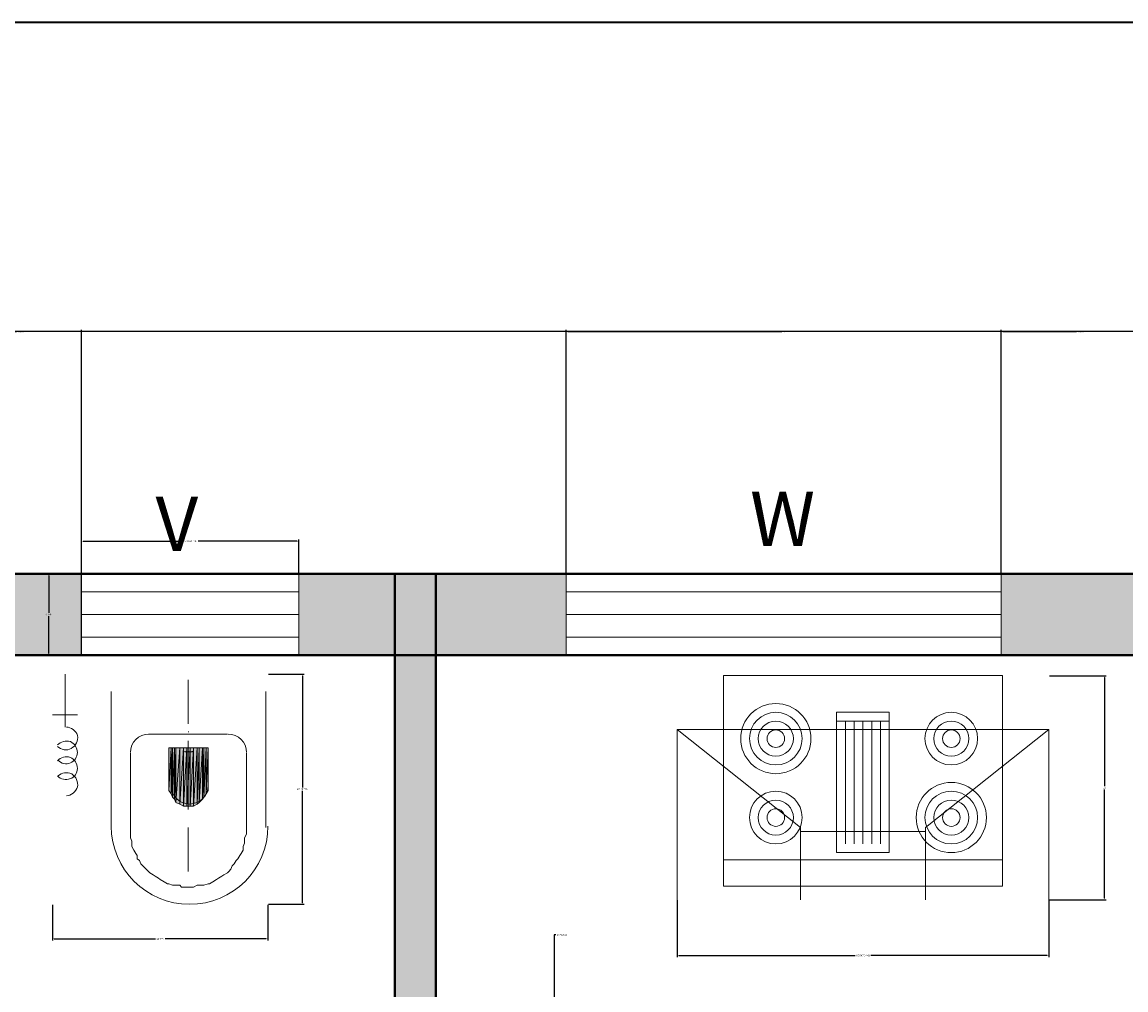
# Model space of a CAD drawing. Units: inches. Extents: x 25176543 to 25177243, y 80295576 to 80296086.
# Tile 9 of 11: x 25176879 to 25177000, y 80295979 to 80296086. Entities that reach past the tile are written whole.
import ezdxf

# ---------------------------------------------------------------- set-up
doc = ezdxf.new("R2010")
doc.units = ezdxf.units.IN
doc.header["$MEASUREMENT"] = 0
for name, color, linetype, lineweight in [('A-ANNO-DIMS', 2, 'Continuous', 18), ('A-ANNO-IDEN', 7, 'Continuous', 18), ('A-ANNO-TTLB', 7, 'Continuous', 35), ('A-EQPM', 8, 'Continuous', 18), ('A-FLOR-FIXT', 8, 'Continuous', 18), ('A-GLAZ', 4, 'Continuous', 18), ('A-WALL', 7, 'Continuous', 40), ('A-WALL-PATT', 146, 'Continuous', 13)]:
    doc.layers.add(name, color=color, linetype=linetype, lineweight=lineweight)
doc.styles.get("Standard").update_dxf_attribs({"font": 'arial.ttf'})
doc.dimstyles.get("Standard").update_dxf_attribs({"dimtxt": 0.18, "dimasz": 0.18, "dimexe": 0.18, "dimexo": 0.0625, "dimgap": 0.09, "dimtad": 0, "dimtih": 1, "dimtoh": 1, "dimdec": 4, "dimzin": 0, "dimdsep": 46, "dimtxsty": 'Standard', "dimcen": 0.09, "dimadec": 0, "dimazin": 0, "dimtfac": 1, "dimtdec": 4, "dimtofl": 0, "dimtmove": 0, "dimatfit": 3, "dimfxl": 1, "dimtolj": 1, "dimtzin": 0, "dimarcsym": 0})

# ---------------------------------------------------------------- blocks, each defined once
blk = doc.blocks.new('chimmne')
for p, q in [((17.89, 6.07), (-18.11, 6.07)), ((-18.11, 6.07), (-18.11, -10.43)), ((-6.16, -3.43), (-18.11, 6.07)), ((5.94, -3.43), (17.89, 6.07)), ((17.89, 6.07), (17.89, -10.43)), ((-6.16, -3.43), (-6.16, -10.43)), ((5.94, -3.82), (-6.16, -3.82)), ((5.94, -3.43), (5.94, -10.43))]:
    blk.add_line(p, q)
for points in [[(-13.61, -9.12), (-13.61, 11.28), (13.39, 11.28), (13.39, -9.12)], [(-2.66, -5.87), (-2.66, 7.73), (2.44, 7.73), (2.44, -5.87)]]:
    blk.add_lwpolyline(points, close=True)
for points in [[(-2.66, 6.88), (2.44, 6.88)], [(-1.81, 6.88), (-1.81, -5.02)], [(-0.96, -5.02), (-0.96, 6.88)], [(-0.11, 6.88), (-0.11, -5.02)], [(0.74, -5.02), (0.74, 6.88)], [(1.59, 6.88), (1.59, -5.02)], [(13.39, -6.57), (-13.61, -6.57)]]:
    blk.add_lwpolyline(points)
for centre, radius in [((-8.55, 5.18), 3.4), ((-8.55, 5.18), 2.55), ((8.44, 5.18), 2.55), ((-8.55, 5.18), 1.7), ((8.44, 5.18), 1.7), ((-8.55, 5.18), 0.85), ((8.44, 5.18), 0.85), ((-8.55, -2.47), 2.55), ((8.44, -2.47), 3.4), ((8.44, -2.47), 2.55), ((-8.55, -2.47), 1.7), ((8.44, -2.47), 1.7), ((-8.55, -2.47), 0.85), ((8.44, -2.47), 0.85)]:
    blk.add_circle(centre, radius)
blk = doc.blocks.new('WC-PLAN')
h = blk.add_hatch(color=256)
h.paths.add_polyline_path([(12.84, 17.3), (12.84, 12.59), (13.07, 17.3)])
h.paths.add_polyline_path([(12.84, 12.59), (13.07, 17.3), (13.07, 12.21)])
h = blk.add_hatch(color=256)
h.paths.add_polyline_path([(13.07, 17.3), (13.07, 12.21), (13.22, 17.3)])
h.paths.add_polyline_path([(13.07, 12.21), (13.22, 17.3), (13.22, 11.83)])
h = blk.add_hatch(color=256)
h.paths.add_polyline_path([(13.22, 17.3), (13.22, 11.83), (13.45, 17.3)])
h.paths.add_polyline_path([(13.22, 11.83), (13.45, 17.3), (13.45, 11.61)])
h = blk.add_hatch(color=256)
h.paths.add_polyline_path([(13.45, 17.3), (13.45, 11.61), (13.6, 17.3)])
h.paths.add_polyline_path([(13.45, 11.61), (13.6, 17.3), (13.6, 11.23)])
h = blk.add_hatch(color=256)
h.paths.add_polyline_path([(13.6, 17.3), (13.6, 11.23), (14.06, 17.3)])
h.paths.add_polyline_path([(13.6, 11.23), (14.06, 17.3), (14.06, 11.08)])
h = blk.add_hatch(color=256)
h.paths.add_polyline_path([(14.06, 17.3), (14.06, 11.08), (14.44, 17.3)])
h.paths.add_polyline_path([(14.06, 11.08), (14.44, 17.3), (14.44, 10.85)])
h = blk.add_hatch(color=256)
h.paths.add_polyline_path([(14.44, 17.3), (14.44, 10.85), (14.81, 17.3)])
h.paths.add_polyline_path([(14.44, 10.85), (14.81, 17.3), (14.81, 10.85)])
h = blk.add_hatch(color=256)
h.paths.add_polyline_path([(14.81, 17.3), (14.81, 10.85), (15.19, 17.3)])
h.paths.add_polyline_path([(14.81, 10.85), (15.19, 17.3), (15.19, 10.85)])
h = blk.add_hatch(color=256)
h.paths.add_polyline_path([(15.19, 17.3), (15.19, 10.85), (15.57, 17.3)])
h.paths.add_polyline_path([(15.19, 10.85), (15.57, 17.3), (15.57, 10.85)])
h = blk.add_hatch(color=256)
h.paths.add_polyline_path([(15.57, 17.3), (15.57, 10.85), (15.95, 17.3)])
h.paths.add_polyline_path([(15.57, 10.85), (15.95, 17.3), (15.95, 11.08)])
h = blk.add_hatch(color=256)
h.paths.add_polyline_path([(15.95, 17.3), (15.95, 11.08), (16.18, 17.3)])
h.paths.add_polyline_path([(15.95, 11.08), (16.18, 17.3), (16.18, 11.23)])
h = blk.add_hatch(color=256)
h.paths.add_polyline_path([(16.18, 17.3), (16.18, 11.23), (16.56, 17.3)])
h.paths.add_polyline_path([(16.18, 11.23), (16.56, 17.3), (16.56, 11.61)])
h = blk.add_hatch(color=256)
h.paths.add_polyline_path([(16.56, 17.3), (16.56, 11.61), (16.71, 17.3)])
h.paths.add_polyline_path([(16.56, 11.61), (16.71, 17.3), (16.71, 11.83)])
h = blk.add_hatch(color=256)
h.paths.add_polyline_path([(16.71, 17.3), (16.71, 11.83), (16.94, 17.3)])
h.paths.add_polyline_path([(16.71, 11.83), (16.94, 17.3), (16.94, 12.21)])
h = blk.add_hatch(color=256)
h.paths.add_polyline_path([(16.94, 17.3), (16.94, 12.21), (17.17, 17.3)])
h.paths.add_polyline_path([(16.94, 12.21), (17.17, 17.3), (17.17, 12.59)])
h.paths.add_polyline_path([(17.17, 17.3), (17.17, 12.59), (17.17, 12.97)])
for points in [[(1.37, 25.41), (1.37, 19.57), (1.37, 19.57)], [(14.97, 24.81), (14.97, 19.95), (14.97, 19.95)], [(6.47, 23.52), (6.47, 8.5), (6.47, 8.5)], [(23.54, 23.52), (23.54, 8.5), (23.54, 8.5)], [(2.73, 20.94), (0, 20.94), (0, 20.94)], [(19.29, 18.81), (10.57, 18.81), (10.57, 18.81)], [(14.97, 19.04), (15.04, 19.04), (15.04, 19.04)], [(17.17, 17.3), (12.84, 17.3), (12.84, 17.3)], [(12.84, 17.3), (12.84, 12.97), (12.84, 12.97)], [(14.97, 18.05), (14.97, 10.47), (14.97, 10.47)], [(17.17, 17.3), (17.17, 12.97), (17.17, 12.97)], [(8.59, 16.69), (8.59, 9.48), (8.59, 9.48)], [(14.59, 16.84), (14.59, 16.92), (14.59, 16.92)], [(14.97, 16.84), (14.81, 16.84), (14.59, 16.84)], [(14.97, 16.84), (15.04, 16.92), (15.04, 16.92)], [(15.42, 16.84), (15.19, 16.84), (14.97, 16.84)], [(15.42, 16.84), (15.42, 16.92), (15.42, 16.92)], [(21.41, 16.69), (21.41, 9.48), (21.41, 9.48)], [(21.41, 9.48), (21.41, 8.72), (21.41, 8.12), (21.41, 7.74), (21.19, 7.36), (21.19, 6.98), (21.19, 6.75), (21.04, 6.37), (21.04, 5.99), (20.81, 5.61), (20.66, 5.39), (20.43, 5.01), (20.28, 4.85), (20.05, 4.48), (19.82, 4.25), (19.67, 3.87), (19.44, 3.64), (19.29, 3.49), (18.91, 3.26), (18.68, 3.11), (18.3, 2.88), (18.08, 2.73), (17.7, 2.5), (17.32, 2.28), (17.17, 2.28), (16.71, 2.12), (16.33, 2.12), (15.95, 2.12), (15.57, 1.9), (14.97, 1.9), (14.21, 1.9), (14.06, 2.12), (13.6, 2.12), (13.22, 2.12), (12.84, 2.28), (12.69, 2.28), (12.31, 2.5), (11.86, 2.73), (11.7, 2.88), (11.33, 3.11), (11.1, 3.26), (10.72, 3.49), (10.57, 3.64), (10.34, 3.87), (9.96, 4.25), (9.73, 4.48), (9.58, 4.85), (9.35, 5.01), (9.35, 5.39), (9.2, 5.61), (8.97, 5.99), (8.75, 6.37), (8.75, 6.75), (8.75, 6.98), (8.59, 7.36), (8.59, 7.74), (8.59, 8.12), (8.59, 8.72), (8.59, 9.48)], [(14.97, 8.5), (14.97, 3.64), (14.97, 3.64)]]:
    blk.add_lwpolyline(points)
for points in [[(12.84, 17.3), (12.84, 12.97)], [(12.84, 12.97), (12.84, 17.3), (12.84, 12.59)], [(12.84, 17.3), (12.84, 12.59), (13.07, 17.3)], [(12.84, 12.59), (13.07, 17.3), (13.07, 12.21)], [(13.07, 17.3), (13.07, 12.21), (13.22, 17.3)], [(13.07, 12.21), (13.22, 17.3), (13.22, 11.83)], [(13.22, 17.3), (13.22, 11.83), (13.45, 17.3)], [(13.22, 11.83), (13.45, 17.3), (13.45, 11.61)], [(13.45, 17.3), (13.45, 11.61), (13.6, 17.3)], [(13.45, 11.61), (13.6, 17.3), (13.6, 11.23)], [(13.6, 17.3), (13.6, 11.23), (14.06, 17.3)], [(13.6, 11.23), (14.06, 17.3), (14.06, 11.08)], [(14.06, 17.3), (14.06, 11.08), (14.44, 17.3)], [(14.06, 11.08), (14.44, 17.3), (14.44, 10.85)], [(14.44, 17.3), (14.44, 10.85), (14.81, 17.3)], [(14.44, 10.85), (14.81, 17.3), (14.81, 10.85)], [(14.81, 17.3), (14.81, 10.85), (15.19, 17.3)], [(14.81, 10.85), (15.19, 17.3), (15.19, 10.85)], [(15.19, 17.3), (15.19, 10.85), (15.57, 17.3)], [(15.19, 10.85), (15.57, 17.3), (15.57, 10.85)], [(15.57, 17.3), (15.57, 10.85), (15.95, 17.3)], [(15.57, 10.85), (15.95, 17.3), (15.95, 11.08)], [(15.95, 17.3), (15.95, 11.08), (16.18, 17.3)], [(15.95, 11.08), (16.18, 17.3), (16.18, 11.23)], [(16.18, 17.3), (16.18, 11.23), (16.56, 17.3)], [(16.18, 11.23), (16.56, 17.3), (16.56, 11.61)], [(16.56, 17.3), (16.56, 11.61), (16.71, 17.3)], [(16.56, 11.61), (16.71, 17.3), (16.71, 11.83)], [(16.71, 17.3), (16.71, 11.83), (16.94, 17.3)], [(16.71, 11.83), (16.94, 17.3), (16.94, 12.21)], [(16.94, 17.3), (16.94, 12.21), (17.17, 17.3)], [(16.94, 12.21), (17.17, 17.3), (17.17, 12.59)], [(17.17, 17.3), (17.17, 12.59), (17.17, 12.97)], [(17.17, 12.59), (17.17, 17.3), (17.17, 17.3)]]:
    blk.add_lwpolyline(points, close=True)
for points, knots in [([(0.53, 17.45), (0.91, 17.07), (1.59, 16.92), (2.05, 17.22), (2.05, 17.22), (2.58, 17.52), (2.88, 18.05), (2.73, 18.66), (2.73, 18.66), (2.58, 19.19), (2.05, 19.57), (1.52, 19.57)], [0, 0, 0, 0, 0.083333, 0.083333, 0.083333, 0.083334, 0.166667, 0.166667, 0.166667, 0.166668, 1, 1, 1, 1]), ([(0.61, 15.93), (0.91, 15.55), (1.52, 15.4), (1.97, 15.63), (1.97, 15.63), (2.43, 15.78), (2.73, 16.31), (2.73, 16.76), (2.73, 16.76), (2.73, 17.3), (2.43, 17.75), (1.97, 17.98), (1.97, 17.98), (1.44, 18.13), (0.91, 17.98), (0.53, 17.6)], [0, 0, 0, 0, 0.0625, 0.0625, 0.0625, 0.062501, 0.125, 0.125, 0.125, 0.125001, 0.1875, 0.1875, 0.1875, 0.187501, 1, 1, 1, 1]), ([(0.53, 14.19), (0.91, 13.81), (1.44, 13.65), (1.97, 13.88), (1.97, 13.88), (2.43, 14.03), (2.73, 14.49), (2.73, 15.02), (2.73, 15.02), (2.73, 15.55), (2.43, 16.01), (1.97, 16.23), (1.97, 16.23), (1.44, 16.39), (0.91, 16.23), (0.53, 15.85)], [0, 0, 0, 0, 0.0625, 0.0625, 0.0625, 0.062501, 0.125, 0.125, 0.125, 0.125001, 0.1875, 0.1875, 0.1875, 0.187501, 1, 1, 1, 1]), ([(1.52, 11.99), (2.05, 11.99), (2.58, 12.44), (2.73, 12.97), (2.73, 12.97), (2.88, 13.5), (2.58, 14.11), (2.12, 14.41), (2.12, 14.41), (1.59, 14.64), (0.99, 14.56), (0.61, 14.19)], [0, 0, 0, 0, 0.083333, 0.083333, 0.083333, 0.083334, 0.166667, 0.166667, 0.166667, 0.166668, 1, 1, 1, 1]), ([(13.07, 13.12), (13.07, 11.99), (13.98, 11.08), (15.12, 11.08), (15.12, 11.08), (16.26, 11.08), (17.17, 11.99), (17.17, 13.12)], [0, 0, 0, 0, 0.125, 0.125, 0.125, 0.125001, 1, 1, 1, 1]), ([(6.47, 8.65), (6.47, 3.87), (10.34, 0), (15.12, 0), (15.12, 0), (19.9, 0), (23.77, 3.87), (23.77, 8.65)], [0, 0, 0, 0, 0.125, 0.125, 0.125, 0.125001, 1, 1, 1, 1])]:
    blk.add_open_spline(points, degree=3, knots=knots)
for points in [[(10.64, 18.81), (9.5, 18.81), (8.59, 17.9), (8.59, 16.76)], [(21.41, 16.76), (21.41, 17.9), (20.5, 18.81), (19.37, 18.81)]]:
    blk.add_open_spline(points, degree=3)
blk = doc.blocks.new('VENT-WIN-24IN')
for p, q in [((0, 9), (0, 0)), ((0, 9), (24, 9)), ((24, 0), (24, 9)), ((0, 7), (24, 7)), ((0, 4.5), (24, 4.5)), ((24, 2), (0, 2)), ((0, 0), (24, 0))]:
    blk.add_line(p, q)
blk = doc.blocks.new('*D22')
at = {"layer": 'A-ANNO-DIMS', "color": 0, "lineweight": -2, "transparency": 16777216}
for p, q in [((25176885.19, 80296025.36), (25176885.19, 80296029.08)), ((25176885.37, 80296028.9), (25176896.28, 80296028.9)), ((25176909.01, 80296028.9), (25176898.09, 80296028.9)), ((25176909.19, 80296025.36), (25176909.19, 80296029.08))]:
    blk.add_line(p, q, dxfattribs=at)
at = {"layer": 'A-ANNO-DIMS', "color": 0, "transparency": 16777216}
for points in [[(25176885.37, 80296028.93), (25176885.37, 80296028.87), (25176885.19, 80296028.9)], [(25176909.01, 80296028.93), (25176909.01, 80296028.87), (25176909.19, 80296028.9)]]:
    blk.add_solid(points, dxfattribs=at)
at = {"layer": 'Defpoints', "color": 0, "transparency": 16777216}
for p in [(25176885.19, 80296028.9), (25176885.19, 80296025.3), (25176909.19, 80296025.3)]:
    blk.add_point(p, dxfattribs=at)
at = {"layer": 'A-ANNO-DIMS', "color": 0, "transparency": 16777216, "insert": (25176897.19, 80296028.9), "char_height": 0.18, "attachment_point": 5}
blk.add_mtext('\\A1;VENT 24 TYP.', dxfattribs=at)
blk = doc.blocks.new('*D23')
at = {"layer": 'A-ANNO-DIMS', "color": 0, "lineweight": -2, "transparency": 16777216}
for p, q in [((25176885.12, 80296025.3), (25176881.41, 80296025.3)), ((25176881.59, 80296025.12), (25176881.59, 80296020.98)), ((25176881.59, 80296016.48), (25176881.59, 80296020.62)), ((25176885.12, 80296016.3), (25176881.41, 80296016.3))]:
    blk.add_line(p, q, dxfattribs=at)
at = {"layer": 'A-ANNO-DIMS', "color": 0, "transparency": 16777216}
for points in [[(25176881.56, 80296025.12), (25176881.62, 80296025.12), (25176881.59, 80296025.3)], [(25176881.56, 80296016.48), (25176881.62, 80296016.48), (25176881.59, 80296016.3)]]:
    blk.add_solid(points, dxfattribs=at)
at = {"layer": 'Defpoints', "color": 0, "transparency": 16777216}
for p in [(25176885.19, 80296025.3), (25176881.59, 80296016.3), (25176885.19, 80296016.3)]:
    blk.add_point(p, dxfattribs=at)
at = {"layer": 'A-ANNO-DIMS', "color": 0, "transparency": 16777216, "insert": (25176881.59, 80296020.8), "char_height": 0.18, "attachment_point": 5}
blk.add_mtext('\\A1;9 TYP.', dxfattribs=at)
blk = doc.blocks.new('*D34')
at = {"layer": 'A-ANNO-DIMS', "color": 0, "lineweight": -2, "transparency": 16777216}
for p, q in [((25176905.84, 80296014.19), (25176909.77, 80296014.19)), ((25176909.59, 80296014.01), (25176909.59, 80296001.67)), ((25176909.59, 80295988.96), (25176909.59, 80296001.3)), ((25176905.84, 80295988.78), (25176909.77, 80295988.78))]:
    blk.add_line(p, q, dxfattribs=at)
at = {"layer": 'A-ANNO-DIMS', "color": 0, "transparency": 16777216}
for points in [[(25176909.56, 80296014.01), (25176909.62, 80296014.01), (25176909.59, 80296014.19)], [(25176909.56, 80295988.96), (25176909.62, 80295988.96), (25176909.59, 80295988.78)]]:
    blk.add_solid(points, dxfattribs=at)
at = {"layer": 'Defpoints', "color": 0, "transparency": 16777216}
for p in [(25176905.77, 80296014.19), (25176909.59, 80296014.19), (25176905.77, 80295988.78)]:
    blk.add_point(p, dxfattribs=at)
at = {"layer": 'A-ANNO-DIMS', "color": 0, "transparency": 16777216, "insert": (25176909.59, 80296001.49), "char_height": 0.18, "attachment_point": 5}
blk.add_mtext('\\A1;WC 25 TYP.', dxfattribs=at)
blk = doc.blocks.new('*D35')
at = {"layer": 'A-ANNO-DIMS', "color": 0, "lineweight": -2, "transparency": 16777216}
for p, q in [((25176882.01, 80295988.72), (25176882.01, 80295984.79)), ((25176905.77, 80295988.72), (25176905.77, 80295984.79)), ((25176882.19, 80295984.97), (25176893.36, 80295984.97)), ((25176905.59, 80295984.97), (25176894.42, 80295984.97))]:
    blk.add_line(p, q, dxfattribs=at)
at = {"layer": 'A-ANNO-DIMS', "color": 0, "transparency": 16777216}
for points in [[(25176882.19, 80295985), (25176882.19, 80295984.94), (25176882.01, 80295984.97)], [(25176905.59, 80295985), (25176905.59, 80295984.94), (25176905.77, 80295984.97)]]:
    blk.add_solid(points, dxfattribs=at)
at = {"layer": 'Defpoints', "color": 0, "transparency": 16777216}
for p in [(25176882.01, 80295988.78), (25176905.77, 80295988.78), (25176905.77, 80295984.97)]:
    blk.add_point(p, dxfattribs=at)
at = {"layer": 'A-ANNO-DIMS', "color": 0, "transparency": 16777216, "insert": (25176893.89, 80295984.97), "char_height": 0.18, "attachment_point": 5}
blk.add_mtext('\\A1;24 TYP.', dxfattribs=at)
blk = doc.blocks.new('*D46')
at = {"layer": 'A-ANNO-DIMS', "color": 0, "lineweight": -2, "transparency": 16777216}
for p, q in [((25176950.94, 80295989.23), (25176950.94, 80295982.95)), ((25176991.98, 80295989.23), (25176991.98, 80295982.95)), ((25176951.12, 80295983.13), (25176970.6, 80295983.13)), ((25176991.8, 80295983.13), (25176972.33, 80295983.13))]:
    blk.add_line(p, q, dxfattribs=at)
at = {"layer": 'A-ANNO-DIMS', "color": 0, "transparency": 16777216}
for points in [[(25176951.12, 80295983.16), (25176951.12, 80295983.1), (25176950.94, 80295983.13)], [(25176991.8, 80295983.16), (25176991.8, 80295983.1), (25176991.98, 80295983.13)]]:
    blk.add_solid(points, dxfattribs=at)
at = {"layer": 'Defpoints', "color": 0, "transparency": 16777216}
for p in [(25176950.94, 80295989.29), (25176991.98, 80295989.29), (25176991.98, 80295983.13)]:
    blk.add_point(p, dxfattribs=at)
at = {"layer": 'A-ANNO-DIMS', "color": 0, "transparency": 16777216, "insert": (25176971.46, 80295983.13), "char_height": 0.18, "attachment_point": 5}
blk.add_mtext('\\A1;COOKTOP 41', dxfattribs=at)
blk = doc.blocks.new('*D47')
at = {"layer": 'A-ANNO-DIMS', "color": 0, "lineweight": -2, "transparency": 16777216}
for p, q in [((25176992.04, 80296014.03), (25176998.32, 80296014.03)), ((25176998.14, 80296013.85), (25176998.14, 80296001.84)), ((25176998.14, 80295989.47), (25176998.14, 80296001.48)), ((25176992.04, 80295989.29), (25176998.32, 80295989.29))]:
    blk.add_line(p, q, dxfattribs=at)
at = {"layer": 'A-ANNO-DIMS', "color": 0, "transparency": 16777216}
for points in [[(25176998.11, 80296013.85), (25176998.17, 80296013.85), (25176998.14, 80296014.03)], [(25176998.11, 80295989.47), (25176998.17, 80295989.47), (25176998.14, 80295989.29)]]:
    blk.add_solid(points, dxfattribs=at)
at = {"layer": 'Defpoints', "color": 0, "transparency": 16777216}
for p in [(25176991.98, 80296014.03), (25176998.14, 80296014.03), (25176991.98, 80295989.29)]:
    blk.add_point(p, dxfattribs=at)
at = {"layer": 'A-ANNO-DIMS', "color": 0, "transparency": 16777216, "insert": (25176998.14, 80296001.66), "char_height": 0.18, "attachment_point": 5}
blk.add_mtext('\\A1;25', dxfattribs=at)
blk = doc.blocks.new('*D48')
at = {"layer": 'A-ANNO-DIMS', "color": 0, "lineweight": -2, "transparency": 16777216}
for p, q in [((25176625.3, 80295890.36), (25176625.3, 80296052.23)), ((25176625.48, 80296052.05), (25176875.16, 80296052.05)), ((25177125.62, 80296052.05), (25176875.95, 80296052.05)), ((25177125.8, 80296025.36), (25177125.8, 80296052.23))]:
    blk.add_line(p, q, dxfattribs=at)
at = {"layer": 'A-ANNO-DIMS', "color": 0, "transparency": 16777216}
for points in [[(25176625.48, 80296052.08), (25176625.48, 80296052.02), (25176625.3, 80296052.05)], [(25177125.62, 80296052.08), (25177125.62, 80296052.02), (25177125.8, 80296052.05)]]:
    blk.add_solid(points, dxfattribs=at)
at = {"layer": 'Defpoints', "color": 0, "transparency": 16777216}
for p in [(25177125.8, 80296052.05), (25177125.8, 80296025.3), (25176625.3, 80295890.3)]:
    blk.add_point(p, dxfattribs=at)
at = {"layer": 'A-ANNO-DIMS', "color": 0, "transparency": 16777216, "insert": (25176875.55, 80296052.05), "char_height": 0.18, "attachment_point": 5}
blk.add_mtext('\\A1;500.5', dxfattribs=at)
blk = doc.blocks.new('*D65')
at = {"layer": 'A-ANNO-DIMS', "color": 0, "lineweight": -2, "transparency": 16777216}
for p, q in [((25176938.71, 80296025.36), (25176938.71, 80296052.23)), ((25176938.89, 80296052.05), (25176962.49, 80296052.05)), ((25176986.53, 80296052.05), (25176962.94, 80296052.05)), ((25176986.71, 80296025.36), (25176986.71, 80296052.23))]:
    blk.add_line(p, q, dxfattribs=at)
at = {"layer": 'A-ANNO-DIMS', "color": 0, "transparency": 16777216}
for points in [[(25176938.89, 80296052.08), (25176938.89, 80296052.02), (25176938.71, 80296052.05)], [(25176986.53, 80296052.08), (25176986.53, 80296052.02), (25176986.71, 80296052.05)]]:
    blk.add_solid(points, dxfattribs=at)
at = {"layer": 'Defpoints', "color": 0, "transparency": 16777216}
for p in [(25176986.71, 80296052.05), (25176938.71, 80296025.3), (25176986.71, 80296025.3)]:
    blk.add_point(p, dxfattribs=at)
at = {"layer": 'A-ANNO-DIMS', "color": 0, "transparency": 16777216, "insert": (25176962.71, 80296052.05), "char_height": 0.18, "attachment_point": 5}
blk.add_mtext('\\A1;48', dxfattribs=at)
blk = doc.blocks.new('*D66')
at = {"layer": 'A-ANNO-DIMS', "color": 0, "lineweight": -2, "transparency": 16777216}
for p, q in [((25176986.71, 80296025.36), (25176986.71, 80296052.23)), ((25176986.89, 80296052.05), (25176995.05, 80296052.05)), ((25177004.12, 80296052.05), (25176995.96, 80296052.05)), ((25177004.3, 80296025.36), (25177004.3, 80296052.23))]:
    blk.add_line(p, q, dxfattribs=at)
at = {"layer": 'A-ANNO-DIMS', "color": 0, "transparency": 16777216}
for points in [[(25176986.89, 80296052.08), (25176986.89, 80296052.02), (25176986.71, 80296052.05)], [(25177004.12, 80296052.08), (25177004.12, 80296052.02), (25177004.3, 80296052.05)]]:
    blk.add_solid(points, dxfattribs=at)
at = {"layer": 'Defpoints', "color": 0, "transparency": 16777216}
for p in [(25177004.3, 80296052.05), (25176986.71, 80296025.3), (25177004.3, 80296025.3)]:
    blk.add_point(p, dxfattribs=at)
at = {"layer": 'A-ANNO-DIMS', "color": 0, "transparency": 16777216, "insert": (25176995.51, 80296052.05), "char_height": 0.18, "attachment_point": 5}
blk.add_mtext('\\A1;17.587', dxfattribs=at)
blk = doc.blocks.new('*D68')
at = {"layer": 'A-ANNO-DIMS', "color": 0, "lineweight": -2, "transparency": 16777216}
for p, q in [((25176871.8, 80296016.36), (25176871.8, 80296052.23)), ((25176871.98, 80296052.05), (25176878.04, 80296052.05)), ((25176885.01, 80296052.05), (25176878.95, 80296052.05)), ((25176885.19, 80296016.36), (25176885.19, 80296052.23))]:
    blk.add_line(p, q, dxfattribs=at)
at = {"layer": 'A-ANNO-DIMS', "color": 0, "transparency": 16777216}
for points in [[(25176871.98, 80296052.08), (25176871.98, 80296052.02), (25176871.8, 80296052.05)], [(25176885.01, 80296052.08), (25176885.01, 80296052.02), (25176885.19, 80296052.05)]]:
    blk.add_solid(points, dxfattribs=at)
at = {"layer": 'Defpoints', "color": 0, "transparency": 16777216}
for p in [(25176885.19, 80296052.05), (25176871.8, 80296016.3), (25176885.19, 80296016.3)]:
    blk.add_point(p, dxfattribs=at)
at = {"layer": 'A-ANNO-DIMS', "color": 0, "transparency": 16777216, "insert": (25176878.49, 80296052.05), "char_height": 0.18, "attachment_point": 5}
blk.add_mtext('\\A1;13.386', dxfattribs=at)
blk = doc.blocks.new('*D79')
at = {"layer": 'A-ANNO-DIMS', "color": 0, "lineweight": -2, "transparency": 16777216}
for p, q in [((25176937.39, 80295985.41), (25176937.33, 80295956.64)), ((25176937.57, 80295985.41), (25176937.39, 80295985.41)), ((25176937.14, 80295908.2), (25176937.32, 80295908.2)), ((25176937.23, 80295908.11), (25176937.23, 80295908.29))]:
    blk.add_line(p, q, dxfattribs=at)
at = {"layer": 'A-ANNO-DIMS', "color": 0, "transparency": 16777216}
blk.add_solid([(25176937.3, 80295956.64), (25176937.36, 80295956.64), (25176937.33, 80295956.46)], dxfattribs=at)
at = {"layer": 'Defpoints', "color": 0, "transparency": 16777216}
for p in [(25176937.33, 80295956.46), (25176937.23, 80295908.2)]:
    blk.add_point(p, dxfattribs=at)
at = {"layer": 'A-ANNO-DIMS', "color": 0, "transparency": 16777216, "insert": (25176938.24, 80295985.41), "char_height": 0.18, "attachment_point": 5}
blk.add_mtext('\\A1;2X R48.26', dxfattribs=at)

msp = doc.modelspace()

# ---------------------------------------------------------------- hatches: boundary and pattern name
at = {"layer": 'A-WALL-PATT'}
h = msp.add_hatch(color=256, dxfattribs=at)
h.dxf.hatch_style = 1
h.paths.add_polyline_path([(25176695.189, 80296025.3022), (25176658.8016, 80296025.3022), (25176658.8016, 80296016.3022), (25176695.189, 80296016.3022)])
h.paths.add_polyline_path([(25176810.3016, 80296025.3022), (25176755.189, 80296025.3022), (25176755.189, 80296016.3022), (25176810.3016, 80296016.3022)])
h.paths.add_polyline_path([(25176819.3016, 80296016.3022), (25176814.8016, 80296016.3022), (25176814.8016, 80295965.3022), (25176819.3016, 80295965.3022)], flags=17)
h.paths.add_polyline_path([(25176828.0421, 80296025.3022), (25176819.3016, 80296025.3022), (25176819.3016, 80296016.3022), (25176828.0421, 80296016.3022)])
h.paths.add_polyline_path([(25176867.3016, 80296025.3022), (25176852.0421, 80296025.3022), (25176852.0421, 80296016.3022), (25176867.3016, 80296016.3022)])
h.paths.add_polyline_path([(25176885.1873, 80296025.3022), (25176876.3016, 80296025.3022), (25176876.3016, 80296016.3022), (25176885.1873, 80296016.3022)])
h.paths.add_polyline_path([(25176919.8016, 80296025.3022), (25176909.1873, 80296025.3022), (25176909.1873, 80296016.3022), (25176919.8016, 80296016.3022)])
h.paths.add_polyline_path([(25176924.3016, 80296016.3022), (25176919.8016, 80296016.3022), (25176919.8016, 80295890.3022), (25176904.8016, 80295890.3022), (25176904.8016, 80295885.8022), (25176967.3016, 80295885.8022), (25176967.3016, 80295890.3022), (25176924.3016, 80295890.3022)])
h.paths.add_polyline_path([(25176924.3016, 80296025.3022), (25176919.8016, 80296025.3022), (25176919.8016, 80296016.3022), (25176924.3016, 80296016.3022)])
h.paths.add_polyline_path([(25176938.7147, 80296025.3022), (25176924.3016, 80296025.3022), (25176924.3016, 80296016.3022), (25176938.7147, 80296016.3022)])
h.paths.add_polyline_path([(25176871.8016, 80296016.3022), (25176867.3016, 80296016.3022), (25176867.3016, 80295932.3022), (25176819.3016, 80295932.3022), (25176819.3016, 80295933.3022), (25176814.8016, 80295933.3022), (25176814.8016, 80295932.3022), (25176814.8016, 80295927.3022), (25176819.3016, 80295927.3022), (25176819.3016, 80295927.8022), (25176867.3016, 80295927.8022), (25176867.3016, 80295885.8022), (25176871.8016, 80295885.8022), (25176872.8016, 80295885.8022), (25176872.8016, 80295890.3022), (25176871.8016, 80295890.3022)])
h.paths.add_polyline_path([(25177004.3016, 80296025.3022), (25176986.7147, 80296025.3022), (25176986.7147, 80296016.3022), (25177004.3016, 80296016.3022)])
h.paths.add_polyline_path([(25177035.845, 80296025.3022), (25177013.3016, 80296025.3022), (25177013.3016, 80296016.3022), (25177035.845, 80296016.3022)])
h.paths.add_polyline_path([(25177008.8016, 80296016.3022), (25177004.3016, 80296016.3022), (25177004.3016, 80295890.3022), (25177003.3016, 80295890.3022), (25177003.3016, 80295885.8022), (25177004.3016, 80295885.8022), (25177004.3016, 80295885.3022), (25177008.8016, 80295885.3022)])
h.paths.add_polyline_path([(25177116.8016, 80296025.3022), (25177095.845, 80296025.3022), (25177095.845, 80296016.3022), (25177116.8016, 80296016.3022)])
h.paths.add_polyline_path([(25177125.8016, 80296016.3022), (25177116.8016, 80296016.3022), (25177116.8016, 80295971.1334), (25177121.3016, 80295971.1334), (25177125.8016, 80295971.1334)])
h.paths.add_polyline_path([(25177116.8016, 80295848.3022), (25177013.3016, 80295848.3022), (25177013.3016, 80295843.8022), (25177116.8016, 80295843.8022)])
h.paths.add_polyline_path([(25177125.8016, 80295911.1334), (25177116.8016, 80295911.1334), (25177116.8016, 80295848.3022), (25177125.8016, 80295848.3022)])
h.paths.add_polyline_path([(25177008.8016, 80295802.3022), (25177004.3016, 80295802.3022), (25177004.3016, 80295676.8022), (25177008.8016, 80295676.8022)])
h.paths.add_polyline_path([(25176658.8016, 80295705.5694), (25176649.8016, 80295705.5694), (25176649.8016, 80295676.8022), (25176658.8016, 80295676.8022)])
h.paths.add_polyline_path([(25176658.8016, 80295798.3022), (25176649.8016, 80295798.3022), (25176649.8016, 80295765.5694), (25176654.3016, 80295765.5694), (25176658.8016, 80295765.5694)])
h.paths.add_polyline_path([(25176833.3016, 80295807.3022), (25176658.8016, 80295807.3022), (25176658.8016, 80295802.8022), (25176833.3016, 80295802.8022)])
h.paths.add_polyline_path([(25176842.3016, 80295761.3022), (25176837.8016, 80295761.3022), (25176837.8016, 80295676.8022), (25176842.3016, 80295676.8022)])
h.paths.add_polyline_path([(25176649.8016, 80295807.3022), (25176629.8016, 80295807.3022), (25176629.8016, 80295885.8022), (25176649.8016, 80295885.8022), (25176649.8016, 80295890.3022), (25176625.3016, 80295890.3022), (25176625.3016, 80295802.8022), (25176649.8016, 80295802.8022)])
h.paths.add_polyline_path([(25176810.3016, 80295890.3022), (25176658.8016, 80295890.3022), (25176658.8016, 80295885.8022), (25176810.3016, 80295885.8022)])
h.paths.add_polyline_path([(25176658.8016, 80295922.9263), (25176649.8016, 80295922.9263), (25176649.8016, 80295890.3022), (25176658.8016, 80295890.3022)])
h.paths.add_polyline_path([(25176658.8016, 80296016.3022), (25176649.8016, 80296016.3022), (25176649.8016, 80295982.9263), (25176654.3016, 80295982.9263), (25176658.8016, 80295982.9263)])

# ---------------------------------------------------------------- linework, layer by layer
at = {"layer": 'A-ANNO-TTLB'}
msp.add_lwpolyline([(25176542.8973, 80296086.2335), (25177242.9194, 80296086.2335), (25177242.9194, 80295575.9501), (25176542.8973, 80295575.9501)], close=True, dxfattribs=at)
at = {"layer": 'A-GLAZ'}
for p, q in [((25176885.1873, 80296025.3022), (25176885.1873, 80296020.8022)), ((25176938.7147, 80296025.3022), (25176938.7147, 80296016.3022)), ((25176986.7147, 80296025.3022), (25176938.7147, 80296025.3022)), ((25176938.7147, 80296025.3022), (25176938.7147, 80296016.3022)), ((25176986.7147, 80296016.3022), (25176986.7147, 80296025.3022)), ((25176986.7147, 80296023.3022), (25176938.7147, 80296023.3022)), ((25176885.1873, 80296020.8022), (25176885.1873, 80296020.8022)), ((25176938.7147, 80296020.8022), (25176986.7147, 80296020.8022)), ((25176938.7147, 80296018.3022), (25176986.7147, 80296018.3022)), ((25176938.7147, 80296016.3022), (25176986.7147, 80296016.3022))]:
    msp.add_line(p, q, dxfattribs=at)
at = {"layer": 'A-WALL'}
for p, q in [((25176649.8016, 80296025.3022), (25177125.8016, 80296025.3022)), ((25176919.8016, 80296025.3022), (25176919.8016, 80295890.3022)), ((25176924.3016, 80296025.3022), (25176924.3016, 80295890.3022)), ((25176649.8016, 80296016.3022), (25177125.8016, 80296016.3022))]:
    msp.add_line(p, q, dxfattribs=at)

# ---------------------------------------------------------------- block references
at = {"layer": 'A-EQPM', "xscale": 1.14, "yscale": 1.14, "zscale": 1.14}
msp.add_blockref('chimmne', (25176971.5894, 80296001.1789), dxfattribs=at)
at = {"layer": 'A-FLOR-FIXT'}
msp.add_blockref('WC-PLAN', (25176882.0091, 80295988.781), dxfattribs=at)
at = {"layer": 'A-GLAZ', "rotation": 180}
msp.add_blockref('VENT-WIN-24IN', (25176909.1873, 80296025.3024), dxfattribs=at)

# ---------------------------------------------------------------- texts
at = {"layer": 'A-ANNO-IDEN', "char_height": 6, "attachment_point": 1}
for s, width, insert in [('W', 24.139595, (25176958.9933, 80296034.3523)), ('V', 12.911449, (25176893.3684, 80296033.8121))]:
    msp.add_mtext_dynamic_manual_height_columns(s, width=width, gutter_width=1, heights=[0], dxfattribs=dict(at, insert=insert))

# ---------------------------------------------------------------- dimensions: what is measured, and where the dimension line sits
at = {"layer": 'A-ANNO-DIMS'}
for base, p1, p2, override, picture, middle in [((25177125.8016, 80296052.0522), (25176625.3016, 80295890.3022), (25177125.8016, 80296025.3022), {"dimdec": 1, "dimlfac": 1, "dimrnd": 0, "dimzin": 0, "dimdsep": 46, "dimlunit": 2}, '*D48', (25176875.5516, 80296052.0522)), ((25176885.1873, 80296052.0522), (25176871.8016, 80296016.3022), (25176885.1873, 80296016.3022), {"dimdec": 3, "dimlfac": 1, "dimrnd": 0, "dimzin": 0, "dimdsep": 46, "dimlunit": 2}, '*D68', (25176878.4944, 80296052.0522)), ((25176986.7147, 80296052.0522), (25176938.7147, 80296025.3022), (25176986.7147, 80296025.3022), {"dimdec": 0, "dimlfac": 1, "dimrnd": 0, "dimzin": 0, "dimdsep": 46, "dimlunit": 2}, '*D65', (25176962.7147, 80296052.0522)), ((25177004.3016, 80296052.0522), (25176986.7147, 80296025.3022), (25177004.3016, 80296025.3022), {"dimdec": 3, "dimlfac": 1, "dimrnd": 0, "dimzin": 0, "dimdsep": 46, "dimlunit": 2}, '*D66', (25176995.5081, 80296052.0522))]:
    dim = msp.add_linear_dim(base=base, p1=p1, p2=p2, dimstyle='Standard', override=override, dxfattribs=at)
    dim.commit()
    dim.dimension.update_dxf_attribs({"geometry": picture, "text_midpoint": middle})
for base, p1, p2, angle, text, picture, middle in [((25176885.1873, 80296028.9022), (25176909.1873, 80296025.3022), (25176885.1873, 80296025.3022), 180, 'VENT <> TYP.', '*D22', (25176897.1873, 80296028.9022)), ((25176881.5873, 80296016.3022), (25176885.1873, 80296025.3022), (25176885.1873, 80296016.3022), 270, '<> TYP.', '*D23', (25176881.5873, 80296020.8022)), ((25176909.5868, 80296014.193), (25176905.7749, 80295988.7809), (25176905.7749, 80296014.193), 90, 'WC <> TYP.', '*D34', (25176909.5868, 80296001.4869))]:
    dim = msp.add_linear_dim(base=base, p1=p1, p2=p2, angle=angle, text=text, dimstyle='Standard', override={"dimdec": 0, "dimlfac": 1, "dimrnd": 0, "dimzin": 0, "dimdsep": 46, "dimlunit": 2}, dxfattribs=at)
    dim.commit()
    dim.dimension.update_dxf_attribs({"geometry": picture, "text_midpoint": middle})
dim = msp.add_linear_dim(base=(25176998.1375, 80296014.0341), p1=(25176991.9815, 80295989.289), p2=(25176991.9815, 80296014.0341), angle=90, dimstyle='Standard', override={"dimdec": 0, "dimlfac": 1, "dimrnd": 0, "dimzin": 0, "dimdsep": 46, "dimlunit": 2}, dxfattribs=at)
dim.commit()
dim.dimension.update_dxf_attribs({"geometry": '*D47', "text_midpoint": (25176998.1375, 80296001.6615)})
for base, p1, p2, text, picture, middle in [((25176991.9815, 80295983.133), (25176950.9415, 80295989.289), (25176991.9815, 80295989.289), 'COOKTOP <>', '*D46', (25176971.4615, 80295983.133)), ((25176905.7749, 80295984.969), (25176882.0092, 80295988.7809), (25176905.7749, 80295988.7809), '<> TYP.', '*D35', (25176893.8921, 80295984.969))]:
    dim = msp.add_linear_dim(base=base, p1=p1, p2=p2, text=text, dimstyle='Standard', override={"dimdec": 0, "dimlfac": 1, "dimrnd": 0, "dimzin": 0, "dimdsep": 46, "dimlunit": 2}, dxfattribs=at)
    dim.commit()
    dim.dimension.update_dxf_attribs({"geometry": picture, "text_midpoint": middle})
dim = msp.add_radius_dim(center=(25176937.225, 80295908.2018), mpoint=(25176937.326, 80295956.4572), text='2X <>', dimstyle='Standard', override={"dimdec": 2, "dimlfac": 1, "dimrnd": 0, "dimzin": 0, "dimdsep": 46, "dimlunit": 2}, dxfattribs=at)
dim.commit()
dim.dimension.update_dxf_attribs({"geometry": '*D79', "text_midpoint": (25176938.2413, 80295985.4104), "dimtype": 164})

doc.saveas('drawing.dxf')
